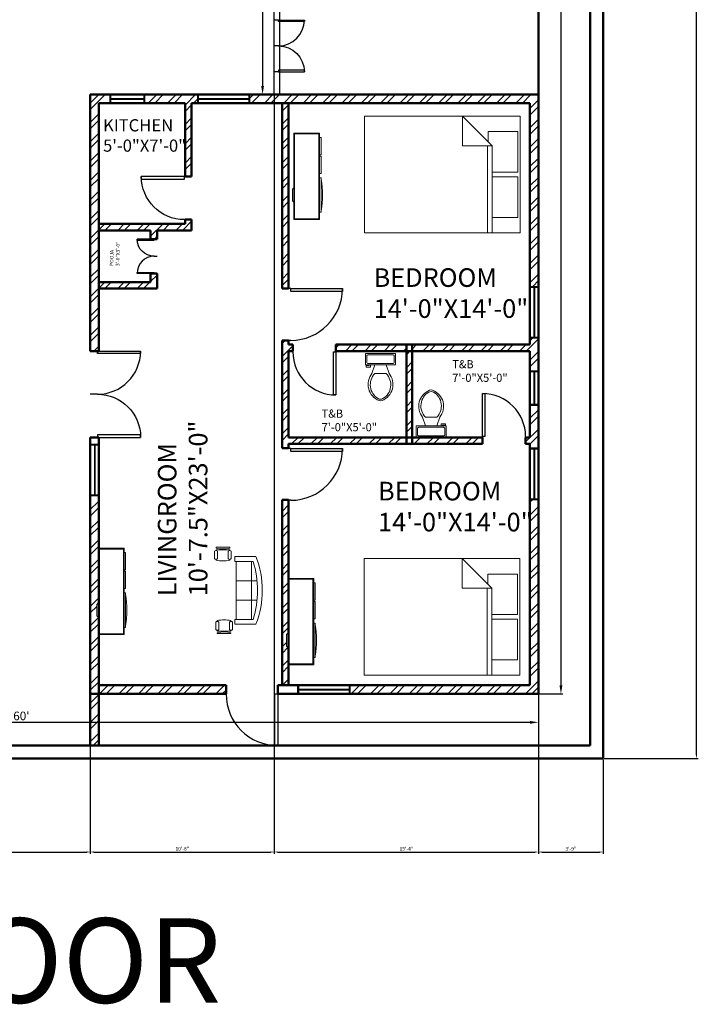
# Model space of a CAD drawing. Units: inches. Extents: x -12550 to 6516, y 1273 to 18700.
# Tile 9 of 19: x 3538 to 4010, y 1273 to 1958. Entities that reach past the tile are written whole.
import ezdxf

# ---------------------------------------------------------------- set-up
doc = ezdxf.new("R2010")
doc.units = ezdxf.units.IN
for name, color, linetype, lineweight in [('A-ANNO-DIMS', 2, 'Continuous', 18), ('A-ANNO-TEXT', 7, 'Continuous', 25), ('A-AREA-IDEN', 1, 'Continuous', 18), ('A-DOOR', 5, 'Continuous', 25), ('A-EQPM', 4, 'Continuous', 25), ('A-FURN', 8, 'Continuous', 18), ('A-GLAZ', 3, 'Continuous', 25), ('A-WALL', 7, 'Continuous', 50), ('A-WALL-PATT', 8, 'Continuous', 13)]:
    doc.layers.add(name, color=color, linetype=linetype, lineweight=lineweight)
doc.styles.get("Standard").update_dxf_attribs({"font": 'arial.ttf'})
doc.dimstyles.new('ISO-25', dxfattribs={"dimtxt": 2.5, "dimasz": 2.5, "dimexe": 1.25, "dimexo": 0.625, "dimtad": 1, "dimlunit": 4, "dimtxsty": 'Standard', "dimcen": 2.5, "dimadec": 0, "dimazin": 0, "dimtfac": 1, "dimtmove": 0, "dimatfit": 3, "dimfxl": 1, "dimarcsym": 0})
pattern_1 = [(45, (1161.5385, 0), (-6.735192, 6.735192), []), (45, (1166.029, 0), (-6.735192, 6.735192), [])]

# ---------------------------------------------------------------- blocks, each defined once
blk = doc.blocks.new('*U2')
for p, q in [((0, 0), (0, -5)), ((30, 0), (30, -5))]:
    blk.add_line(p, q)
blk.add_lwpolyline([(0, 0), (0, 30), (1.75, 30), (1.75, 0)], close=True)
blk.add_arc((0, 0), 30, 0, 90)
blk = doc.blocks.new('Bed - Queen')
for p, q in [((0, -80.00003), (0, 0)), ((0, 0), (59.99999, 0)), ((59.99999, 0), (59.99999, -80.00003)), ((7.99999, -1.2), (28.79998, -1.2)), ((7.99999, -14.4), (7.99999, -1.2)), ((28.79998, -1.2), (28.79998, -14.4)), ((31.19999, -1.2), (51.99999, -1.2)), ((31.19999, -14.4), (31.19999, -1.2)), ((51.99999, -1.2), (51.99999, -16.4)), ((0, -14.4), (44.8, -14.4)), ((59.99999, -29.6), (44.8, -14.4)), ((44.8, -14.4), (44.8, -29.6)), ((44.8, -16.8), (0, -16.8)), ((51.99999, -16.4), (46.79936, -16.4)), ((44.8, -29.6), (59.99999, -29.6)), ((59.99999, -80.00003), (0, -80.00003))]:
    blk.add_line(p, q)
blk = doc.blocks.new('Toilet - top')
for p, q in [((9.5, -6), (9.5, -2)), ((-10, -8.5), (-8, -8.5)), ((-10, -9.5), (-10, -8.5)), ((-7, -9.5), (-10, -9.5)), ((-8, -8.5), (-8, -8)), ((-7, -8), (-7, -9.5)), ((-4, -8), (-6, -14)), ((4, -8), (6, -14)), ((4, -14), (-4, -14))]:
    blk.add_line(p, q)
blk.add_lwpolyline([(10.5, -8), (10.5, 0), (-10.5, 0), (-10.5, -8)], close=True)
for points in [[(-9.5, -2), (-9.5, -6)], [(8.5, -1), (-8.5, -1)], [(-8.5, -7), (8.5, -7)]]:
    blk.add_lwpolyline(points)
for centre, radius, start, end in [((-8.62, -1.88), 0.884, 81.8699, 188.1301), ((-8.62, -6.12), 0.884, 171.8699, 278.1301), ((8.62, -1.88), 0.884, 351.8699, 98.1301), ((8.62, -6.12), 0.884, 261.8699, 8.1301), ((3.52, -21.58), 12.17, 141.46911, 247.97143), ((4.2, -21.82), 11.33, 136.36773, 238.94682), ((-3.52, -21.58), 12.17, 292.02843, 38.53071), ((-4.2, -21.82), 11.33, 301.05301, 43.63209), ((0, -27.88), 4, 245.73182, 294.26817), ((0, -29), 4, 254.86053, 285.13947)]:
    blk.add_arc(centre, radius, start, end)
blk = doc.blocks.new('Entertainment Center')
for p, q in [((-4, 0), (-5, -1)), ((4, 0), (-4, 0)), ((5, -1), (4, 0)), ((-17, -19), (-17, -1)), ((-17, -1), (43, -1)), ((-16.5, -18.5), (-16.5, -1.5)), ((-16.5, -1.5), (42.5, -1.5)), ((42.5, -1.5), (42.5, -18.5)), ((43, -1), (43, -19)), ((43, -19), (-17, -19)), ((42.5, -18.5), (-16.5, -18.5)), ((-12, -20), (-12, -19)), ((12, -20), (-12, -20)), ((12, -19), (12, -20)), ((15, -20), (15, -19)), ((27, -20), (15, -20)), ((27, -19), (27, -20)), ((28, -20), (28, -19)), ((40, -20), (28, -20)), ((40, -19), (40, -20))]:
    blk.add_line(p, q)
blk.add_arc((0, 40), 61, 259.6111, 280.3889)
blk = doc.blocks.new('Sofa - Roundback 7 ft.')
for p, q in [((-36.000027, -34), (-36.000027, -11.4696)), ((-12.00002, -32.4421), (-12.00003, -6.5971)), ((11.99997, -32.4421), (11.99998, -6.5971)), ((35.99998, -34), (35.99998, -11.4696)), ((-35.999844, -13.3819), (35.9998, -13.3819)), ((-36.000027, -32.4421), (35.99998, -32.4421))]:
    blk.add_line(p, q)
for points in [[(-36.000027, -34), (-42.000027, -34), (-42.000027, -8)], [(41.99998, -8), (41.99998, -34), (35.99998, -34)]]:
    blk.add_lwpolyline(points)
for centre, radius, start, end in [((0, -114.25), 114.25, 68.43141, 111.5686), ((-0.00001, -127.1968), 121.1968, 72.72033, 107.2797)]:
    blk.add_arc(centre, radius, start, end)
blk = doc.blocks.new('Chair - Desk')
for p, q in [((-8.5, 0), (-8.5, -1)), ((-8.5, 0), (8.5, 0)), ((8.5, 0), (8.5, -1)), ((-10.5, -5), (-10.5, -14)), ((-8.5, -3), (-8.5, -4)), ((-8.5, -3), (8.5, -3)), ((-6.5, -14), (-6.5, -5)), ((-2, -3), (-2, -1.9355)), ((2, -1.9576), (2, -3)), ((6.5, -5), (6.5, -14)), ((8.5, -3), (8.5, -4)), ((10.5, -14), (10.5, -5)), ((-8.5, -15), (-8.5, -16)), ((8.5, -15), (8.5, -16))]:
    blk.add_line(p, q)
for centre, radius, start, end in [((-8.5, -6.5), 2.5, 36.8699, 143.1301), ((0, 34.625), 36.625, 256.5803, 283.4197), ((8.5, -6.5), 2.5, 36.8699, 143.1301), ((-8.5, -12.5), 2.5, 216.8699, 323.1301), ((0, 19.625), 36.625, 256.5803, 283.4197), ((8.5, -12.5), 2.5, 216.8699, 323.1301)]:
    blk.add_arc(centre, radius, start, end)
blk = doc.blocks.new('*D28')
at = {"layer": 'A-ANNO-DIMS', "color": 0, "lineweight": -2, "transparency": 16777216}
for p, q in [((3714.6, 2056.25), (3705.89, 2056.25)), ((3707.14, 2050.25), (3707.14, 1912.25)), ((3714.6, 1906.25), (3705.89, 1906.25))]:
    blk.add_line(p, q, dxfattribs=at)
at = {"layer": 'A-ANNO-DIMS', "color": 0, "transparency": 16777216}
for points in [[(3706.14, 2050.25), (3708.14, 2050.25), (3707.14, 2056.25)], [(3706.14, 1912.25), (3708.14, 1912.25), (3707.14, 1906.25)]]:
    blk.add_solid(points, dxfattribs=at)
at = {"layer": 'Defpoints', "color": 0, "transparency": 16777216}
for p in [(3715.23, 2056.25), (3707.14, 1906.25), (3715.23, 1906.25)]:
    blk.add_point(p, dxfattribs=at)
at = {"layer": 'A-ANNO-DIMS', "color": 0, "transparency": 16777216, "insert": (3703.45, 1981.25), "char_height": 6, "attachment_point": 5, "rotation": 90}
blk.add_mtext('12\'-6"', dxfattribs=at)
blk = doc.blocks.new('*D30')
at = {"layer": 'A-ANNO-DIMS', "color": 0, "lineweight": -2, "transparency": 16777216}
for p, q in [((3899.85, 2473.25), (3916.1, 2473.25)), ((3914.85, 2467.25), (3914.85, 1495.25)), ((3899.85, 1489.25), (3916.1, 1489.25))]:
    blk.add_line(p, q, dxfattribs=at)
at = {"layer": 'A-ANNO-DIMS', "color": 0, "transparency": 16777216}
for points in [[(3913.85, 2467.25), (3915.85, 2467.25), (3914.85, 2473.25)], [(3913.85, 1495.25), (3915.85, 1495.25), (3914.85, 1489.25)]]:
    blk.add_solid(points, dxfattribs=at)
at = {"layer": 'Defpoints', "color": 0, "transparency": 16777216}
for p in [(3899.23, 2473.25), (3899.23, 1489.25), (3914.85, 1489.25)]:
    blk.add_point(p, dxfattribs=at)
at = {"layer": 'A-ANNO-DIMS', "color": 0, "transparency": 16777216, "insert": (3911.16, 1981.25), "char_height": 6, "attachment_point": 5, "rotation": 90}
blk.add_mtext("82'", dxfattribs=at)
blk = doc.blocks.new('*D31')
at = {"layer": 'A-ANNO-DIMS', "color": 0, "lineweight": -2, "transparency": 16777216}
for p, q in [((3179.23, 1488.62), (3179.23, 1468.21)), ((3899.23, 1488.62), (3899.23, 1468.21)), ((3893.23, 1469.46), (3185.23, 1469.46))]:
    blk.add_line(p, q, dxfattribs=at)
at = {"layer": 'A-ANNO-DIMS', "color": 0, "transparency": 16777216}
for points in [[(3185.23, 1470.46), (3185.23, 1468.46), (3179.23, 1469.46)], [(3893.23, 1470.46), (3893.23, 1468.46), (3899.23, 1469.46)]]:
    blk.add_solid(points, dxfattribs=at)
at = {"layer": 'Defpoints', "color": 0, "transparency": 16777216}
for p in [(3179.23, 1489.25), (3899.23, 1489.25), (3179.23, 1469.46)]:
    blk.add_point(p, dxfattribs=at)
at = {"layer": 'A-ANNO-DIMS', "color": 0, "transparency": 16777216, "insert": (3539.23, 1473.15), "char_height": 6, "attachment_point": 5}
blk.add_mtext("60'", dxfattribs=at)
blk = doc.blocks.new('WIN-3FT')
for p, q in [((0, 0), (0, 6)), ((0, 6), (36.02, 6)), ((36.02, 0), (0, 0)), ((0.5, 0), (0.5, 6)), ((35.52, 3.2), (0.5, 3.2)), ((35.52, 2.8), (0.5, 2.8)), ((35.52, 6), (35.52, 0)), ((36.02, 6), (36.02, 0))]:
    blk.add_line(p, q)
blk = doc.blocks.new('WIN-2FT')
for p, q in [((0, 0), (0, 24.02)), ((0, 24.02), (6, 24.02)), ((0, 23.52), (6, 23.52)), ((2.8, 0.5), (2.8, 23.52)), ((3.2, 0.5), (3.2, 23.52)), ((6, 24.02), (6, 0)), ((6, 0.5), (0, 0.5)), ((6, 0), (0, 0))]:
    blk.add_line(p, q)
blk = doc.blocks.new('*D104')
at = {"layer": 'A-ANNO-DIMS', "color": 0, "lineweight": -2, "transparency": 16777216}
for p, q in [((3944.85, 2518.25), (4010.48, 2518.25)), ((4009.23, 1446.75), (4009.23, 2515.75)), ((3944.85, 1444.25), (4010.48, 1444.25))]:
    blk.add_line(p, q, dxfattribs=at)
at = {"layer": 'A-ANNO-DIMS', "color": 0, "transparency": 16777216}
for points in [[(4008.81, 2515.75), (4009.64, 2515.75), (4009.23, 2518.25)], [(4008.81, 1446.75), (4009.64, 1446.75), (4009.23, 1444.25)]]:
    blk.add_solid(points, dxfattribs=at)
at = {"layer": 'Defpoints', "color": 0, "transparency": 16777216}
for p in [(3944.23, 2518.25), (4009.23, 2518.25), (3944.23, 1444.25)]:
    blk.add_point(p, dxfattribs=at)
at = {"layer": 'A-ANNO-DIMS', "color": 0, "transparency": 16777216, "insert": (4007.33, 1981.25), "char_height": 2.5, "attachment_point": 5, "rotation": 90}
blk.add_mtext('89\'-6"', dxfattribs=at)
blk = doc.blocks.new('*D106')
at = {"layer": 'A-ANNO-DIMS', "color": 0, "lineweight": -2, "transparency": 16777216}
for p, q in [((3179.23, 1488.62), (3179.23, 1378)), ((3587.23, 1488.62), (3587.23, 1378)), ((3181.73, 1379.25), (3584.73, 1379.25))]:
    blk.add_line(p, q, dxfattribs=at)
at = {"layer": 'A-ANNO-DIMS', "color": 0, "transparency": 16777216}
for points in [[(3181.73, 1379.66), (3181.73, 1378.83), (3179.23, 1379.25)], [(3584.73, 1379.66), (3584.73, 1378.83), (3587.23, 1379.25)]]:
    blk.add_solid(points, dxfattribs=at)
at = {"layer": 'Defpoints', "color": 0, "transparency": 16777216}
for p in [(3179.23, 1489.25), (3587.23, 1489.25), (3587.23, 1379.25)]:
    blk.add_point(p, dxfattribs=at)
at = {"layer": 'A-ANNO-DIMS', "color": 0, "transparency": 16777216, "insert": (3383.23, 1381.15), "char_height": 2.5, "attachment_point": 5}
blk.add_mtext('34\'-0"', dxfattribs=at)
blk = doc.blocks.new('*D107')
at = {"layer": 'A-ANNO-DIMS', "color": 0, "lineweight": -2, "transparency": 16777216}
for p, q in [((3715.23, 1905.62), (3715.23, 1378)), ((3587.23, 1488.62), (3587.23, 1378)), ((3589.73, 1379.25), (3712.73, 1379.25))]:
    blk.add_line(p, q, dxfattribs=at)
at = {"layer": 'A-ANNO-DIMS', "color": 0, "transparency": 16777216}
for points in [[(3589.73, 1379.66), (3589.73, 1378.83), (3587.23, 1379.25)], [(3712.73, 1379.66), (3712.73, 1378.83), (3715.23, 1379.25)]]:
    blk.add_solid(points, dxfattribs=at)
at = {"layer": 'Defpoints', "color": 0, "transparency": 16777216}
for p in [(3715.23, 1906.25), (3587.23, 1489.25), (3715.23, 1379.25)]:
    blk.add_point(p, dxfattribs=at)
at = {"layer": 'A-ANNO-DIMS', "color": 0, "transparency": 16777216, "insert": (3651.23, 1381.15), "char_height": 2.5, "attachment_point": 5}
blk.add_mtext('10\'-8"', dxfattribs=at)
blk = doc.blocks.new('*D108')
at = {"layer": 'A-ANNO-DIMS', "color": 0, "lineweight": -2, "transparency": 16777216}
for p, q in [((3715.23, 1905.62), (3715.23, 1378)), ((3899.23, 1905.62), (3899.23, 1378)), ((3717.73, 1379.25), (3896.73, 1379.25))]:
    blk.add_line(p, q, dxfattribs=at)
at = {"layer": 'A-ANNO-DIMS', "color": 0, "transparency": 16777216}
for points in [[(3717.73, 1379.66), (3717.73, 1378.83), (3715.23, 1379.25)], [(3896.73, 1379.66), (3896.73, 1378.83), (3899.23, 1379.25)]]:
    blk.add_solid(points, dxfattribs=at)
at = {"layer": 'Defpoints', "color": 0, "transparency": 16777216}
for p in [(3715.23, 1906.25), (3899.23, 1906.25), (3899.23, 1379.25)]:
    blk.add_point(p, dxfattribs=at)
at = {"layer": 'A-ANNO-DIMS', "color": 0, "transparency": 16777216, "insert": (3807.23, 1381.15), "char_height": 2.5, "attachment_point": 5}
blk.add_mtext('15\'-4"', dxfattribs=at)
blk = doc.blocks.new('*D109')
at = {"layer": 'A-ANNO-DIMS', "color": 0, "lineweight": -2, "transparency": 16777216}
for p, q in [((3899.23, 1488.62), (3899.23, 1378)), ((3944.23, 1443.62), (3944.23, 1378)), ((3901.73, 1379.25), (3941.73, 1379.25))]:
    blk.add_line(p, q, dxfattribs=at)
at = {"layer": 'A-ANNO-DIMS', "color": 0, "transparency": 16777216}
for points in [[(3901.73, 1379.66), (3901.73, 1378.83), (3899.23, 1379.25)], [(3941.73, 1379.66), (3941.73, 1378.83), (3944.23, 1379.25)]]:
    blk.add_solid(points, dxfattribs=at)
at = {"layer": 'Defpoints', "color": 0, "transparency": 16777216}
for p in [(3899.23, 1489.25), (3944.23, 1444.25), (3944.23, 1379.25)]:
    blk.add_point(p, dxfattribs=at)
at = {"layer": 'A-ANNO-DIMS', "color": 0, "transparency": 16777216, "insert": (3921.73, 1381.15), "char_height": 2.5, "attachment_point": 5}
blk.add_mtext('3\'-9"', dxfattribs=at)

msp = doc.modelspace()

# ---------------------------------------------------------------- hatches: boundary and pattern name
at = {"layer": 'A-WALL-PATT'}
h = msp.add_hatch(dxfattribs=at)
h.set_pattern_fill('ANSI32', color=256)
h.set_pattern_definition(pattern_1)
h.paths.add_polyline_path([(3600.985, 1906.247), (3587.227, 1906.247), (3587.227, 1727.747), (3592.227, 1727.747), (3593.227, 1727.747), (3593.227, 1900.247), (3600.985, 1900.247)])
h = msp.add_hatch(dxfattribs=at)
h.set_pattern_fill('ANSI32', color=256)
h.set_pattern_definition(pattern_1)
h.paths.add_polyline_path([(3662.066, 1906.247), (3625.002, 1906.247), (3625.002, 1900.247), (3653.227, 1900.247), (3653.227, 1849.247), (3657.727, 1849.247), (3657.727, 1900.247), (3662.066, 1900.247)])
h = msp.add_hatch(dxfattribs=at)
h.set_pattern_fill('ANSI32', color=256)
h.set_pattern_definition(pattern_1)
h.paths.add_polyline_path([(3899.227, 1906.247), (3720.727, 1906.247), (3698.084, 1906.247), (3698.084, 1900.247), (3720.727, 1900.247), (3893.227, 1900.247), (3893.227, 1772.747), (3899.227, 1772.747)])
h = msp.add_hatch(dxfattribs=at)
h.set_pattern_fill('ANSI32', color=256)
h.set_pattern_definition(pattern_1)
h.paths.add_polyline_path([(3725.227, 1900.247), (3720.727, 1900.247), (3720.727, 1771.247), (3725.227, 1771.247)])
h = msp.add_hatch(dxfattribs=at)
h.set_pattern_fill('ANSI32', color=256)
h.set_pattern_definition(pattern_1)
h.paths.add_polyline_path([(3657.727, 1819.247), (3653.227, 1819.247), (3653.227, 1816.247), (3593.227, 1816.247), (3593.227, 1811.747), (3629.227, 1811.747), (3629.227, 1805.747), (3631.727, 1805.747), (3633.727, 1805.747), (3633.727, 1811.747), (3657.727, 1811.747)])
h = msp.add_hatch(dxfattribs=at)
h.set_pattern_fill('ANSI32', color=256)
h.set_pattern_definition(pattern_1)
h.paths.add_polyline_path([(3633.727, 1781.747), (3631.727, 1781.747), (3629.227, 1781.747), (3629.227, 1775.747), (3593.227, 1775.747), (3593.227, 1771.247), (3633.727, 1771.247)])
h = msp.add_hatch(dxfattribs=at)
h.set_pattern_fill('ANSI32', color=256)
h.set_pattern_definition(pattern_1)
h.paths.add_polyline_path([(3725.227, 1727.747), (3728.227, 1727.747), (3728.227, 1732.247), (3725.227, 1732.247), (3725.227, 1735.247), (3720.727, 1735.247), (3720.727, 1660.247), (3725.227, 1660.247), (3725.227, 1663.247), (3728.18, 1663.247), (3807.227, 1663.247), (3807.227, 1667.747), (3728.18, 1667.747), (3725.227, 1667.747)])
h = msp.add_hatch(dxfattribs=at)
h.set_pattern_fill('ANSI32', color=256)
h.set_pattern_definition(pattern_1)
h.paths.add_polyline_path([(3899.227, 1736.73), (3893.227, 1736.73), (3893.227, 1732.247), (3890.227, 1732.247), (3811.227, 1732.247), (3811.227, 1727.747), (3890.227, 1727.747), (3893.227, 1727.747), (3893.227, 1714.042), (3899.227, 1714.042)])
h = msp.add_hatch(dxfattribs=at)
h.set_pattern_fill('ANSI32', color=256)
h.set_pattern_definition(pattern_1)
h.paths.add_polyline_path([(3807.227, 1732.247), (3758.227, 1732.247), (3758.227, 1727.747), (3807.227, 1727.747)], flags=17)
h = msp.add_hatch(dxfattribs=at)
h.set_pattern_fill('ANSI32', color=256)
h.set_pattern_definition(pattern_1)
h.paths.add_polyline_path([(3811.227, 1727.747), (3807.227, 1727.747), (3807.227, 1667.747), (3811.227, 1667.747)])
h = msp.add_hatch(dxfattribs=at)
h.set_pattern_fill('ANSI32', color=256)
h.set_pattern_definition(pattern_1)
h.paths.add_polyline_path([(3899.227, 1690.024), (3893.227, 1690.024), (3893.227, 1667.747), (3890.227, 1667.747), (3890.227, 1663.247), (3893.227, 1663.247), (3893.227, 1660.369), (3899.227, 1660.369)])
h = msp.add_hatch(dxfattribs=at)
h.set_pattern_fill('ANSI32', color=256)
h.set_pattern_definition(pattern_1)
h.paths.add_polyline_path([(3860.227, 1667.747), (3811.227, 1667.747), (3811.227, 1663.247), (3860.227, 1663.247)])
h = msp.add_hatch(dxfattribs=at)
h.set_pattern_fill('ANSI32', color=256)
h.set_pattern_definition(pattern_1)
h.paths.add_polyline_path([(3681.727, 1495.247), (3593.227, 1495.247), (3593.227, 1530.559), (3592.727, 1530.559), (3592.727, 1542.559), (3591.727, 1543.559), (3591.727, 1551.559), (3592.727, 1552.559), (3592.727, 1590.559), (3592.964, 1627.032), (3587.227, 1627.032), (3587.227, 1489.247), (3681.727, 1489.247)])
h = msp.add_hatch(dxfattribs=at)
h.set_pattern_fill('ANSI32', color=256)
h.set_pattern_definition(pattern_1)
h.paths.add_polyline_path([(3720.727, 1623.947), (3720.727, 1495.247), (3725.227, 1495.247), (3725.227, 1509.575), (3724.727, 1509.575), (3724.727, 1521.575), (3723.727, 1522.575), (3723.727, 1530.575), (3724.727, 1531.575), (3724.727, 1569.575), (3725.225, 1623.947)])
h = msp.add_hatch(dxfattribs=at)
h.set_pattern_fill('ANSI32', color=256)
h.set_pattern_definition(pattern_1)
h.paths.add_polyline_path([(3899.227, 1624.352), (3893.227, 1624.352), (3893.227, 1495.247), (3767.813, 1495.247), (3767.813, 1489.247), (3899.227, 1489.247)])
h = msp.add_hatch(dxfattribs=at)
h.set_pattern_fill('ANSI32', color=256)
h.set_pattern_definition(pattern_1)
h.paths.add_polyline_path([(3593.227, 1489.247), (3587.227, 1489.247), (3587.227, 1453.247), (3593.227, 1453.247)])

# ---------------------------------------------------------------- linework, layer by layer
at = {"layer": 'A-EQPM'}
for p, q in [((3715.227, 1906.247), (3715.227, 2056.247)), ((3719.227, 1906.247), (3719.227, 2056.247)), ((3899.227, 2056.247), (3899.227, 1906.247)), ((3899.227, 1906.247), (3715.227, 1906.247))]:
    msp.add_line(p, q, dxfattribs=at)
at = {"layer": 'A-WALL'}
for p, q in [((3944.227, 2518.247), (3944.227, 1444.247)), ((3935.227, 2509.247), (3935.227, 1453.247)), ((3899.227, 1489.247), (3899.227, 2060.923)), ((3935.227, 1489.247), (3935.227, 2060.923)), ((3720.727, 1906.247), (3587.227, 1906.247)), ((3587.227, 1727.747), (3587.227, 1906.247)), ((3899.227, 1906.247), (3720.727, 1906.247)), ((3653.227, 1900.247), (3593.227, 1900.247)), ((3593.227, 1727.747), (3593.227, 1900.247)), ((3653.227, 1849.247), (3653.227, 1900.247)), ((3720.727, 1900.247), (3657.727, 1900.247)), ((3657.727, 1849.247), (3657.727, 1900.247)), ((3893.227, 1900.247), (3720.727, 1900.247)), ((3720.727, 1771.247), (3720.727, 1900.247)), ((3725.227, 1771.247), (3725.227, 1900.247)), ((3893.227, 1732.247), (3893.227, 1900.247)), ((3653.227, 1849.247), (3657.727, 1849.247)), ((3653.227, 1816.247), (3593.227, 1816.247)), ((3653.227, 1816.247), (3653.227, 1819.247)), ((3657.727, 1819.247), (3653.227, 1819.247)), ((3657.727, 1811.747), (3657.727, 1819.247)), ((3657.727, 1816.247), (3657.727, 1819.247)), ((3629.227, 1811.747), (3593.227, 1811.747)), ((3629.227, 1805.747), (3629.227, 1811.747)), ((3657.727, 1811.747), (3633.727, 1811.747)), ((3633.727, 1805.747), (3633.727, 1811.747)), ((3629.227, 1805.747), (3633.727, 1805.747)), ((3629.227, 1775.747), (3629.227, 1781.747)), ((3633.727, 1781.747), (3629.227, 1781.747)), ((3633.727, 1771.247), (3633.727, 1781.747)), ((3633.727, 1775.747), (3633.727, 1781.747)), ((3629.227, 1775.747), (3593.227, 1775.747)), ((3633.727, 1771.247), (3593.227, 1771.247)), ((3720.727, 1771.247), (3725.227, 1771.247)), ((3720.727, 1660.247), (3720.727, 1735.247)), ((3725.227, 1735.247), (3720.727, 1735.247)), ((3725.227, 1732.247), (3725.227, 1735.247)), ((3725.227, 1732.247), (3725.227, 1735.247)), ((3725.227, 1732.247), (3725.227, 1735.247)), ((3725.227, 1732.247), (3725.227, 1735.247)), ((3593.227, 1727.747), (3587.227, 1727.747)), ((3728.227, 1732.247), (3725.227, 1732.247)), ((3728.227, 1727.747), (3725.227, 1727.747)), ((3725.227, 1667.747), (3725.227, 1727.747)), ((3725.227, 1667.747), (3725.227, 1727.747)), ((3725.227, 1667.747), (3725.227, 1727.747)), ((3725.227, 1727.747), (3728.227, 1727.747)), ((3728.227, 1727.747), (3728.227, 1732.247)), ((3890.227, 1732.247), (3758.227, 1732.247)), ((3758.227, 1732.247), (3758.227, 1727.747)), ((3890.227, 1727.747), (3758.227, 1727.747)), ((3807.227, 1663.247), (3807.227, 1732.247)), ((3811.227, 1663.247), (3811.227, 1732.247)), ((3893.227, 1732.247), (3890.227, 1732.247)), ((3893.227, 1732.247), (3890.227, 1732.247)), ((3893.227, 1727.747), (3890.227, 1727.747)), ((3893.227, 1667.747), (3893.227, 1727.747)), ((3593.227, 1667.747), (3587.227, 1667.747)), ((3587.227, 1453.247), (3587.227, 1667.747)), ((3593.227, 1453.247), (3593.227, 1667.747)), ((3728.18, 1667.747), (3725.227, 1667.747)), ((3860.227, 1667.747), (3728.18, 1667.747)), ((3860.227, 1667.747), (3860.227, 1663.247)), ((3893.227, 1667.747), (3890.227, 1667.747)), ((3890.227, 1663.247), (3890.227, 1667.747)), ((3720.727, 1663.247), (3720.727, 1660.247)), ((3720.727, 1660.247), (3725.227, 1660.247)), ((3728.18, 1663.247), (3725.227, 1663.247)), ((3725.227, 1660.247), (3725.227, 1663.247)), ((3725.227, 1660.247), (3725.227, 1663.247)), ((3725.227, 1660.247), (3725.227, 1663.247)), ((3860.227, 1663.247), (3728.18, 1663.247)), ((3893.227, 1663.247), (3890.227, 1663.247)), ((3893.227, 1663.247), (3890.227, 1663.247)), ((3893.227, 1495.247), (3893.227, 1663.247)), ((3720.727, 1495.247), (3720.727, 1624.247)), ((3725.227, 1624.247), (3720.727, 1624.247)), ((3725.227, 1495.247), (3725.227, 1624.247)), ((3681.727, 1495.247), (3593.227, 1495.247)), ((3681.727, 1489.247), (3681.727, 1495.247)), ((3893.227, 1495.247), (3717.727, 1495.247)), ((3720.727, 1495.247), (3717.727, 1495.247)), ((3717.727, 1495.247), (3717.727, 1489.247)), ((3681.727, 1489.247), (3587.227, 1489.247)), ((3899.227, 1489.247), (3717.727, 1489.247)), ((3143.227, 1453.247), (3935.227, 1453.247)), ((3681.727, 1453.247), (3417.727, 1453.247)), ((3134.227, 1444.247), (3944.227, 1444.247))]:
    msp.add_line(p, q, dxfattribs=at)

# ---------------------------------------------------------------- block references
at = {"layer": 'A-DOOR', "xscale": -1}
for p, rotation in [((3652.727, 1849.247), 90), ((3592.227, 1667.747), 270)]:
    msp.add_blockref('*U2', p, dxfattribs=dict(at, rotation=rotation))
at = {"layer": 'A-DOOR'}
for p, xscale, yscale, zscale, rotation in [((3631.727, 1805.747), -0.399999999999997, 0.399999999999997, 0.399999999999997, 90), ((3631.727, 1781.747), 0.399999999999997, 0.399999999999997, 0.399999999999997, 90.00000000000003), ((3726.727, 1771.247), 1.199999999999999, 1.199999999999999, 1.199999999999999, 270), ((3726.727, 1659.947), 1.199999999999999, 1.199999999999999, 1.199999999999999, 270), ((3717.727, 1489.247), 1.199999999999999, 1.199999999999999, 1.199999999999999, 180)]:
    msp.add_blockref('*U2', p, dxfattribs=dict(at, xscale=xscale, yscale=yscale, zscale=zscale, rotation=rotation))
for p, rotation in [((3592.227, 1727.747), 270), ((3758.227, 1727.247), 180)]:
    msp.add_blockref('*U2', p, dxfattribs=dict(at, rotation=rotation))
msp.add_blockref('*U2', (3860.227, 1668.247), dxfattribs=at)
at = {"layer": 'A-EQPM', "yscale": 0.5999999999999954, "zscale": 0.5999999999999954, "rotation": 270}
for p, xscale in [((3718.227, 1958.135), 0.5999999999999954), ((3718.227, 1922.135), -0.5999999999999954)]:
    msp.add_blockref('*U2', p, dxfattribs=dict(at, xscale=xscale))
at = {"layer": 'A-FURN'}
for name, p, xscale, yscale, zscale, rotation in [('Bed - Queen', (3886.407, 1809.994), -1.354827908062564, 1.354827908062564, 1.354827908062564, 270), ('Sofa - Roundback 7 ft.', (3706.946, 1561.265), 0.5595223685495907, 0.5595223685495907, 0.5595223685495907, 270), ('Bed - Queen', (3886.246, 1502.217), -1.354827908062564, 1.354827908062564, 1.354827908062564, 270), ('Chair - Desk', (3680.361, 1531.281), 0.5595223685495907, 0.5595223685495907, 0.5595223685495907, 180)]:
    msp.add_blockref(name, p, dxfattribs=dict(at, xscale=xscale, yscale=yscale, zscale=zscale, rotation=rotation))
for name, p, rotation in [('Entertainment Center', (3727.857, 1836.379), 89.99999999999999), ('Toilet - top', (3824.496, 1667.747), 180), ('Entertainment Center', (3591.727, 1547.559), 89.99999999999999), ('Entertainment Center', (3723.727, 1526.575), 89.99999999999999)]:
    msp.add_blockref(name, p, dxfattribs=dict(at, rotation=rotation))
msp.add_blockref('Toilet - top', (3789.25, 1726.198), dxfattribs=at)
at = {"layer": 'A-FURN', "xscale": 0.5595223685495907, "yscale": 0.5595223685495907, "zscale": 0.5595223685495907}
msp.add_blockref('Chair - Desk', (3679.507, 1591.265), dxfattribs=at)
at = {"layer": 'A-GLAZ'}
for name, p, rotation in [('WIN-2FT', (3600.984, 1906.247), 269.9999999999969), ('WIN-3FT', (3698.083, 1906.247), 180), ('WIN-3FT', (3899.228, 1736.73), 90.00000000000342), ('WIN-2FT', (3899.227, 1714.042), 180), ('WIN-3FT', (3593.228, 1627.032), 90.00000000000058), ('WIN-3FT', (3899.228, 1624.352), 90.0000000000033), ('WIN-3FT', (3767.813, 1495.247), 180)]:
    msp.add_blockref(name, p, dxfattribs=dict(at, rotation=rotation))

# ---------------------------------------------------------------- texts
at = {"layer": 'A-ANNO-TEXT', "insert": (3259.388, 1333.138), "char_height": 58.816, "attachment_point": 1}
msp.add_mtext('2nd FLOOR', dxfattribs=at)
at = {"layer": 'A-AREA-IDEN', "attachment_point": 1}
for s, width, gutter_width, insert, char_height in [('KITCHEN\\P5\'-0"X7\'-0"', 1.29487, 42.422, (3596.107, 1889.124), 8.48435), ('T&B\\P7\'-0"X5\'-0"', 4.19569, 28.328, (3839.149, 1721.465), 5.66556), ('T&B\\P7\'-0"X5\'-0"', 4.19569, 28.328, (3748.24, 1687.107), 5.66556)]:
    msp.add_mtext_dynamic_manual_height_columns(s, width=width, gutter_width=gutter_width, heights=[0], dxfattribs=dict(at, insert=insert, char_height=char_height))
at = {"layer": 'A-AREA-IDEN', "insert": (3600.779, 1787.026), "char_height": 2.5, "attachment_point": 1, "rotation": 89.183853}
msp.add_mtext_dynamic_manual_height_columns('POOJA\\P3\'-0"X3\'-0"', width=0.78585, gutter_width=12.5, heights=[0], dxfattribs=at)
at = {"layer": 'A-AREA-IDEN', "char_height": 12.93169, "attachment_point": 1}
for insert in [(3784.442, 1785.378), (3787.508, 1636.812)]:
    msp.add_mtext('BEDROOM\\P14\'-0"X14\'-0"', dxfattribs=dict(at, insert=insert))
at = {"layer": 'A-AREA-IDEN', "insert": (3634.251, 1557.153), "char_height": 12.93169, "attachment_point": 1, "rotation": 90}
msp.add_mtext('LIVINGROOM\\P10\'-7.5"X23\'-0"', dxfattribs=at)

# ---------------------------------------------------------------- dimensions: what is measured, and where the dimension line sits
at = {"layer": 'A-ANNO-DIMS'}
for base, p1, p2, override, picture, middle in [((4009.227, 2518.247), (3944.227, 1444.247), (3944.227, 2518.247), {"dimdec": 1, "dimlfac": 1, "dimrnd": 0, "dimzin": 1, "dimdsep": 46, "dimlunit": 4, "dimfrac": 2}, '*D104', (4007.326, 1981.247)), ((3914.847, 1489.247), (3899.227, 2473.247), (3899.227, 1489.247), {"dimtxt": 6, "dimasz": 6, "dimclrd": 0, "dimclre": 0, "dimclrt": 0}, '*D30', (3911.159, 1981.247)), ((3707.141, 1906.247), (3715.227, 2056.247), (3715.227, 1906.247), {"dimtxt": 6, "dimasz": 6, "dimclrd": 0, "dimclre": 0, "dimclrt": 0}, '*D28', (3703.452, 1981.247))]:
    dim = msp.add_linear_dim(base=base, p1=p1, p2=p2, angle=90, dimstyle='ISO-25', override=override, dxfattribs=at)
    dim.commit()
    dim.dimension.update_dxf_attribs({"geometry": picture, "text_midpoint": middle})
for base, p1, p2, override, picture, middle in [((3715.227, 1379.247), (3587.227, 1489.247), (3715.227, 1906.247), {"dimdec": 1, "dimlfac": 1, "dimrnd": 0, "dimzin": 1, "dimdsep": 46, "dimlunit": 4, "dimfrac": 2}, '*D107', (3651.227, 1381.149)), ((3899.227, 1379.247), (3715.227, 1906.247), (3899.227, 1906.247), {"dimdec": 1, "dimlfac": 1, "dimrnd": 0, "dimzin": 1, "dimdsep": 46, "dimlunit": 4, "dimfrac": 2}, '*D108', (3807.227, 1381.149)), ((3179.227, 1469.461), (3899.227, 1489.247), (3179.227, 1489.247), {"dimtxt": 6, "dimasz": 6, "dimclrd": 0, "dimclre": 0, "dimclrt": 0}, '*D31', (3539.227, 1473.15)), ((3587.227, 1379.247), (3179.227, 1489.247), (3587.227, 1489.247), {"dimdec": 1, "dimlfac": 1, "dimrnd": 0, "dimzin": 1, "dimdsep": 46, "dimlunit": 4, "dimfrac": 2}, '*D106', (3383.227, 1381.15)), ((3944.227, 1379.247), (3899.227, 1489.247), (3944.227, 1444.247), {"dimdec": 1, "dimlfac": 1, "dimrnd": 0, "dimzin": 1, "dimdsep": 46, "dimlunit": 4, "dimfrac": 2}, '*D109', (3921.727, 1381.15))]:
    dim = msp.add_linear_dim(base=base, p1=p1, p2=p2, dimstyle='ISO-25', override=override, dxfattribs=at)
    dim.commit()
    dim.dimension.update_dxf_attribs({"geometry": picture, "text_midpoint": middle})

doc.saveas('drawing.dxf')
